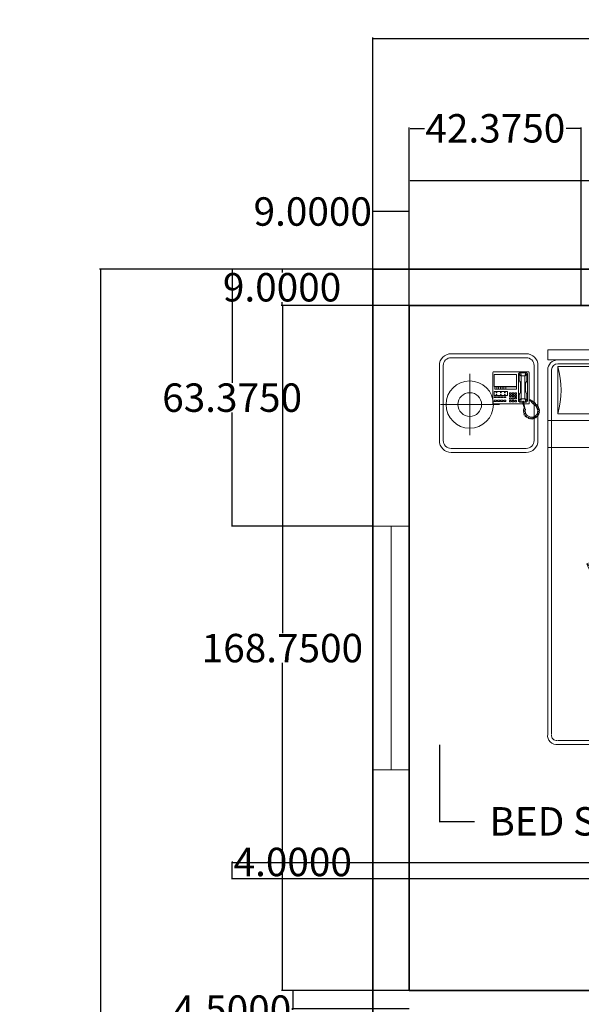
# Model space of a CAD drawing. Units: inches. Extents: x 774 to 2194, y 522 to 1247.
# Tile 4 of 7: x 774 to 912, y 870 to 1112. Entities that reach past the tile are written whole.
import ezdxf

# ---------------------------------------------------------------- set-up
doc = ezdxf.new("R2010")
doc.units = ezdxf.units.IN
for name, color, linetype, lineweight in [('A-ANNO-DIMS', 2, 'Continuous', 13), ('A-FURN', 8, 'Continuous', 18), ('A-GLAZ', 4, 'Continuous', 18), ('A-WALL', 7, 'Continuous', 35)]:
    doc.layers.add(name, color=color, linetype=linetype, lineweight=lineweight)
doc.styles.get("Standard").update_dxf_attribs({"font": 'arial.ttf'})
doc.dimstyles.get("Standard").update_dxf_attribs({"dimtxt": 7, "dimasz": 0.18, "dimexe": 0.18, "dimexo": 0.0625, "dimgap": 0.09, "dimtad": 0, "dimtih": 1, "dimtoh": 1, "dimdec": 4, "dimzin": 0, "dimdsep": 46, "dimtxsty": 'Standard', "dimcen": 0.09, "dimadec": 0, "dimazin": 0, "dimtfac": 1, "dimtdec": 4, "dimtofl": 0, "dimtmove": 0, "dimatfit": 3, "dimfxl": 1, "dimtolj": 1, "dimtzin": 0, "dimarcsym": 0})

# ---------------------------------------------------------------- blocks, each defined once
blk = doc.blocks.new('A$C356F0359')
for p, q in [((0.5489, 2), (2.0492, 2)), ((0.5489, 1.9489), (0.5489, 2)), ((2.0492, 1.9489), (2.0492, 2)), ((0.4398, 1.9801), (0.0598, 1.9801)), ((0.4398, 1.9601), (0.0598, 1.9601)), ((2.0492, 1.9489), (0.5489, 1.9489)), ((2.5283, 1.9801), (2.1483, 1.9801)), ((2.5283, 1.9601), (2.1483, 1.9601)), ((-0.0002, 1.9201), (-0.0002, 1.5401)), ((0.0198, 1.9201), (0.0198, 1.5401)), ((0.4798, 1.5401), (0.4798, 1.9201)), ((0.4998, 1.5401), (0.4998, 1.9201)), ((0.5489, 1.8977), (0.5489, 0.0512)), ((0.5689, 1.8977), (0.5689, 0.0512)), ((1.998, 1.9289), (0.6001, 1.9289)), ((2.0292, 0.0512), (2.0292, 1.8977)), ((2.0492, 0.0512), (2.0492, 1.8977)), ((2.0883, 1.9201), (2.0883, 1.5401)), ((2.1083, 1.9201), (2.1083, 1.5401)), ((2.5683, 1.5401), (2.5683, 1.9201)), ((2.5883, 1.5401), (2.5883, 1.9201)), ((0.1539, 1.5681), (0.1539, 1.8777)), ((0.2725, 1.8879), (0.2702, 1.8856)), ((0.2702, 1.8856), (0.2702, 1.7279)), ((0.2725, 1.8879), (0.4531, 1.8879)), ((0.3913, 1.8753), (0.277, 1.8753)), ((0.277, 1.8753), (0.277, 1.8147)), ((0.3913, 1.8147), (0.3913, 1.8753)), ((0.4016, 1.8787), (0.4062, 1.8845)), ((0.4016, 1.7404), (0.4016, 1.8787)), ((0.4062, 1.881), (0.405, 1.8765)), ((0.405, 1.8765), (0.4153, 1.8662)), ((0.405, 1.8765), (0.405, 1.8456)), ((0.4062, 1.8845), (0.4405, 1.8845)), ((0.4108, 1.8833), (0.4062, 1.881)), ((0.4108, 1.8833), (0.4382, 1.8833)), ((0.4165, 1.8685), (0.4108, 1.8833)), ((0.4153, 1.8662), (0.4165, 1.8685)), ((0.4153, 1.8147), (0.4153, 1.8662)), ((0.4325, 1.8685), (0.4165, 1.8685)), ((0.4325, 1.8685), (0.4382, 1.8833)), ((0.4336, 1.8662), (0.4325, 1.8685)), ((0.4439, 1.8765), (0.4336, 1.8662)), ((0.4336, 1.8147), (0.4336, 1.8662)), ((0.4382, 1.8833), (0.4428, 1.881)), ((0.4405, 1.8845), (0.4462, 1.8787)), ((0.4428, 1.881), (0.4439, 1.8765)), ((0.4439, 1.8765), (0.4439, 1.8456)), ((0.4462, 1.8787), (0.4462, 1.7416)), ((0.4531, 1.8879), (0.4553, 1.8856)), ((0.4553, 1.8856), (0.4553, 1.7279)), ((2.3306, 1.5822), (2.3306, 1.8917)), ((0.277, 1.8147), (0.3913, 1.8147)), ((0.3913, 1.8125), (0.2816, 1.8125)), ((0.2816, 1.8125), (0.2816, 1.801)), ((0.2816, 1.801), (0.3913, 1.801)), ((0.2907, 1.8125), (0.2907, 1.801)), ((0.2999, 1.8125), (0.2999, 1.801)), ((0.309, 1.8125), (0.309, 1.801)), ((0.3182, 1.8125), (0.3182, 1.801)), ((0.3273, 1.8125), (0.3273, 1.801)), ((0.3365, 1.8125), (0.3365, 1.801)), ((0.3913, 1.801), (0.3913, 1.8125)), ((0.405, 1.8456), (0.4073, 1.8399)), ((0.4073, 1.8399), (0.4108, 1.8342)), ((0.4108, 1.8342), (0.4119, 1.8262)), ((0.4119, 1.8262), (0.4119, 1.8147)), ((0.4119, 1.793), (0.4119, 1.8147)), ((0.4153, 1.8147), (0.4153, 1.753)), ((0.4336, 1.8147), (0.4336, 1.753)), ((0.4382, 1.8342), (0.4371, 1.8262)), ((0.4371, 1.8262), (0.4371, 1.8147)), ((0.4371, 1.793), (0.4371, 1.8147)), ((0.4416, 1.8399), (0.4382, 1.8342)), ((0.4439, 1.8456), (0.4416, 1.8399)), ((0.277, 1.7885), (0.277, 1.7679)), ((0.3445, 1.7885), (0.277, 1.7885)), ((0.277, 1.7679), (0.3445, 1.7679)), ((0.2782, 1.7622), (0.2782, 1.7576)), ((0.2896, 1.7622), (0.2782, 1.7622)), ((0.2782, 1.7576), (0.2896, 1.7576)), ((0.2885, 1.7862), (0.2885, 1.7827)), ((0.2919, 1.7862), (0.2885, 1.7862)), ((0.2885, 1.7827), (0.2919, 1.7827)), ((0.2919, 1.7736), (0.2885, 1.7736)), ((0.2885, 1.7736), (0.2885, 1.7702)), ((0.2885, 1.7702), (0.2919, 1.7702)), ((0.2896, 1.7576), (0.2896, 1.7622)), ((0.2919, 1.7827), (0.2919, 1.7862)), ((0.2919, 1.7702), (0.2919, 1.7736)), ((0.2942, 1.7622), (0.2942, 1.7576)), ((0.3056, 1.7622), (0.2942, 1.7622)), ((0.2942, 1.7576), (0.3056, 1.7576)), ((0.3056, 1.7576), (0.3056, 1.7622)), ((0.3125, 1.7862), (0.309, 1.7862)), ((0.309, 1.7862), (0.309, 1.7827)), ((0.309, 1.7827), (0.3125, 1.7827)), ((0.3125, 1.7736), (0.309, 1.7736)), ((0.309, 1.7736), (0.309, 1.7702)), ((0.309, 1.7702), (0.3125, 1.7702)), ((0.3102, 1.7622), (0.3102, 1.7576)), ((0.3216, 1.7622), (0.3102, 1.7622)), ((0.3102, 1.7576), (0.3216, 1.7576)), ((0.3125, 1.7827), (0.3125, 1.7862)), ((0.3125, 1.7702), (0.3125, 1.7736)), ((0.3216, 1.7576), (0.3216, 1.7622)), ((0.3376, 1.7622), (0.3262, 1.7622)), ((0.3262, 1.7622), (0.3262, 1.7576)), ((0.3262, 1.7576), (0.3376, 1.7576)), ((0.333, 1.7862), (0.3296, 1.7862)), ((0.3296, 1.7862), (0.3296, 1.7827)), ((0.3296, 1.7827), (0.333, 1.7827)), ((0.333, 1.7736), (0.3296, 1.7736)), ((0.3296, 1.7736), (0.3296, 1.7702)), ((0.3296, 1.7702), (0.333, 1.7702)), ((0.333, 1.7827), (0.333, 1.7862)), ((0.333, 1.7702), (0.333, 1.7736)), ((0.3376, 1.7576), (0.3376, 1.7622)), ((0.3445, 1.7679), (0.3445, 1.7885)), ((0.3548, 1.7759), (0.3548, 1.7827)), ((0.3548, 1.7827), (0.3639, 1.7827)), ((0.3639, 1.7759), (0.3548, 1.7759)), ((0.3548, 1.7633), (0.3548, 1.7702)), ((0.3548, 1.7702), (0.3639, 1.7702)), ((0.3639, 1.7633), (0.3548, 1.7633)), ((0.3548, 1.7564), (0.3639, 1.7564)), ((0.3548, 1.7496), (0.3548, 1.7564)), ((0.3639, 1.7496), (0.3548, 1.7496)), ((0.3639, 1.7827), (0.3639, 1.7759)), ((0.3639, 1.7702), (0.3639, 1.7633)), ((0.3639, 1.7564), (0.3639, 1.7496)), ((0.3685, 1.7827), (0.3776, 1.7827)), ((0.3685, 1.7759), (0.3685, 1.7827)), ((0.3776, 1.7759), (0.3685, 1.7759)), ((0.3685, 1.7633), (0.3685, 1.7702)), ((0.3685, 1.7702), (0.3776, 1.7702)), ((0.3776, 1.7633), (0.3685, 1.7633)), ((0.3685, 1.7564), (0.3776, 1.7564)), ((0.3685, 1.7496), (0.3685, 1.7564)), ((0.3776, 1.7496), (0.3685, 1.7496)), ((0.3776, 1.7827), (0.3776, 1.7759)), ((0.3776, 1.7702), (0.3776, 1.7633)), ((0.3776, 1.7564), (0.3776, 1.7496)), ((0.3822, 1.7759), (0.3822, 1.7827)), ((0.3822, 1.7827), (0.3913, 1.7827)), ((0.3913, 1.7759), (0.3822, 1.7759)), ((0.3822, 1.7633), (0.3822, 1.7702)), ((0.3822, 1.7702), (0.3913, 1.7702)), ((0.3913, 1.7633), (0.3822, 1.7633)), ((0.3822, 1.7576), (0.3913, 1.7576)), ((0.3822, 1.7507), (0.3822, 1.7576)), ((0.3913, 1.7507), (0.3822, 1.7507)), ((0.3913, 1.7827), (0.3913, 1.7759)), ((0.3913, 1.7702), (0.3913, 1.7633)), ((0.3913, 1.7576), (0.3913, 1.7507)), ((0.405, 1.7736), (0.4073, 1.7793)), ((0.405, 1.7427), (0.405, 1.7736)), ((0.405, 1.7427), (0.4153, 1.753)), ((0.4073, 1.7793), (0.4108, 1.785)), ((0.4108, 1.785), (0.4119, 1.793)), ((0.4165, 1.7507), (0.4108, 1.7359)), ((0.4153, 1.753), (0.4165, 1.7507)), ((0.4325, 1.7507), (0.4165, 1.7507)), ((0.4336, 1.753), (0.4325, 1.7507)), ((0.4325, 1.7507), (0.4382, 1.7359)), ((0.4439, 1.7427), (0.4336, 1.753)), ((0.4382, 1.785), (0.4371, 1.793)), ((0.4416, 1.7793), (0.4382, 1.785)), ((0.4439, 1.7736), (0.4416, 1.7793)), ((0.4439, 1.7427), (0.4439, 1.7736)), ((0.4622, 1.7459), (0.4553, 1.7484)), ((0.3052, 1.7226), (0.0051, 1.7226)), ((0.2702, 1.7279), (0.2725, 1.7256)), ((0.4244, 1.7256), (0.2725, 1.7256)), ((0.2782, 1.745), (0.2896, 1.745)), ((0.2782, 1.7382), (0.2782, 1.745)), ((0.2896, 1.7382), (0.2782, 1.7382)), ((0.2896, 1.745), (0.2896, 1.7382)), ((0.2942, 1.745), (0.3056, 1.745)), ((0.2942, 1.7382), (0.2942, 1.745)), ((0.3056, 1.7382), (0.2942, 1.7382)), ((0.3056, 1.745), (0.3056, 1.7382)), ((0.3102, 1.745), (0.3216, 1.745)), ((0.3102, 1.7382), (0.3102, 1.745)), ((0.3216, 1.7382), (0.3102, 1.7382)), ((0.3216, 1.745), (0.3216, 1.7382)), ((0.3262, 1.7382), (0.3262, 1.745)), ((0.3262, 1.745), (0.3376, 1.745)), ((0.3376, 1.7382), (0.3262, 1.7382)), ((0.3376, 1.745), (0.3376, 1.7382)), ((0.3548, 1.737), (0.3548, 1.7439)), ((0.3548, 1.7439), (0.3639, 1.7439)), ((0.3639, 1.737), (0.3548, 1.737)), ((0.3639, 1.7439), (0.3639, 1.737)), ((0.3685, 1.737), (0.3685, 1.7439)), ((0.3685, 1.7439), (0.3776, 1.7439)), ((0.3776, 1.737), (0.3685, 1.737)), ((0.3776, 1.7439), (0.3776, 1.737)), ((0.3822, 1.7439), (0.3913, 1.7439)), ((0.3822, 1.737), (0.3822, 1.7439)), ((0.3913, 1.737), (0.3822, 1.737)), ((0.3913, 1.7439), (0.3913, 1.737)), ((0.4073, 1.7347), (0.4016, 1.7404)), ((0.4062, 1.7382), (0.405, 1.7427)), ((0.4108, 1.7359), (0.4062, 1.7382)), ((0.4234, 1.7347), (0.4073, 1.7347)), ((0.4108, 1.7359), (0.4234, 1.7359)), ((0.4233, 1.7393), (0.4235, 1.7294)), ((0.4268, 1.7393), (0.4233, 1.7393)), ((0.4235, 1.7294), (0.4263, 1.7179)), ((0.4263, 1.7179), (0.429, 1.707)), ((0.427, 1.697), (0.4265, 1.6915)), ((0.4274, 1.7301), (0.4268, 1.7393)), ((0.427, 1.7359), (0.4382, 1.7359)), ((0.4295, 1.6996), (0.427, 1.697)), ((0.4405, 1.7347), (0.4271, 1.7347)), ((0.429, 1.7227), (0.4274, 1.7301)), ((0.4531, 1.7256), (0.4284, 1.7256)), ((0.429, 1.707), (0.4288, 1.701)), ((0.4288, 1.701), (0.4295, 1.6996)), ((0.4318, 1.7119), (0.429, 1.7227)), ((0.4325, 1.7063), (0.4318, 1.7119)), ((0.4323, 1.7003), (0.4325, 1.7063)), ((0.4364, 1.6973), (0.4323, 1.7003)), ((0.4355, 1.6919), (0.4364, 1.6973)), ((0.4382, 1.7359), (0.4428, 1.7382)), ((0.4462, 1.7416), (0.4405, 1.7347)), ((0.4428, 1.7382), (0.4439, 1.7427)), ((0.4553, 1.7279), (0.4531, 1.7256)), ((0.4553, 1.7439), (0.4604, 1.7425)), ((0.4604, 1.7425), (0.465, 1.7388)), ((0.4654, 1.7427), (0.4622, 1.7459)), ((0.465, 1.7388), (0.4662, 1.7372)), ((0.4678, 1.7405), (0.4654, 1.7427)), ((0.4662, 1.7372), (0.4686, 1.7374)), ((0.4686, 1.7374), (0.4662, 1.735)), ((0.4662, 1.735), (0.4755, 1.7268)), ((0.4721, 1.7421), (0.4678, 1.7405)), ((0.4741, 1.7401), (0.4721, 1.7421)), ((0.4725, 1.7366), (0.4741, 1.7401)), ((0.4753, 1.7388), (0.4725, 1.7366)), ((0.4783, 1.7356), (0.4753, 1.7388)), ((0.4755, 1.7268), (0.4906, 1.7139)), ((0.4759, 1.729), (0.4783, 1.7356)), ((0.4821, 1.7322), (0.4759, 1.729)), ((0.4874, 1.7272), (0.4821, 1.7322)), ((0.4862, 1.7199), (0.4874, 1.7272)), ((0.4914, 1.7231), (0.4862, 1.7199)), ((0.4908, 1.7135), (0.4984, 1.6917)), ((0.4958, 1.7185), (0.4914, 1.7231)), ((0.494, 1.7135), (0.4958, 1.7185)), ((0.501, 1.7142), (0.494, 1.7135)), ((0.4964, 1.7047), (0.5031, 1.7072)), ((0.5038, 1.7049), (0.4964, 1.7047)), ((0.5005, 1.695), (0.5054, 1.6996)), ((0.5031, 1.7072), (0.501, 1.7142)), ((0.5054, 1.6996), (0.5038, 1.7049)), ((2.4819, 1.7366), (2.1818, 1.7366)), ((0.4265, 1.6915), (0.4332, 1.6903)), ((0.4332, 1.6903), (0.4267, 1.6864)), ((0.4267, 1.6864), (0.4272, 1.6801)), ((0.4272, 1.6801), (0.4346, 1.6794)), ((0.4346, 1.6794), (0.4281, 1.6744)), ((0.4281, 1.6744), (0.4311, 1.669)), ((0.4311, 1.669), (0.4381, 1.6704)), ((0.4381, 1.6704), (0.4348, 1.6639)), ((0.4348, 1.6639), (0.4383, 1.6598)), ((0.4367, 1.6774), (0.4355, 1.6919)), ((0.4455, 1.6663), (0.4367, 1.6774)), ((0.4383, 1.6598), (0.4436, 1.6637)), ((0.4436, 1.6637), (0.4427, 1.6575)), ((0.4427, 1.6575), (0.4471, 1.6547)), ((0.4577, 1.6598), (0.4455, 1.6663)), ((0.4471, 1.6547), (0.4526, 1.6593)), ((0.4526, 1.6593), (0.4519, 1.6517)), ((0.4519, 1.6517), (0.4568, 1.6503)), ((0.4568, 1.6503), (0.4598, 1.6565)), ((0.4716, 1.6586), (0.4577, 1.6598)), ((0.4598, 1.6565), (0.4626, 1.6503)), ((0.4626, 1.6503), (0.4665, 1.6498)), ((0.4665, 1.6498), (0.4681, 1.6565)), ((0.4681, 1.6565), (0.4707, 1.6491)), ((0.4707, 1.6491), (0.4751, 1.6503)), ((0.485, 1.6644), (0.4716, 1.6586)), ((0.4751, 1.6503), (0.4753, 1.6565)), ((0.4753, 1.6565), (0.4806, 1.6519)), ((0.4806, 1.6519), (0.4843, 1.6538)), ((0.4843, 1.6538), (0.4836, 1.6607)), ((0.4836, 1.6607), (0.4885, 1.6547)), ((0.4952, 1.6744), (0.485, 1.6644)), ((0.4885, 1.6547), (0.4922, 1.6579)), ((0.4922, 1.6579), (0.4894, 1.6642)), ((0.4894, 1.6642), (0.4959, 1.6614)), ((0.4984, 1.6917), (0.4952, 1.6744)), ((0.4957, 1.6704), (0.5024, 1.6683)), ((0.4989, 1.6642), (0.4957, 1.6704)), ((0.4959, 1.6614), (0.4989, 1.6642)), ((0.5042, 1.673), (0.4987, 1.6792)), ((0.4987, 1.6792), (0.5058, 1.679)), ((0.5068, 1.695), (0.5005, 1.695)), ((0.5008, 1.6871), (0.5079, 1.6892)), ((0.5068, 1.6836), (0.5008, 1.6871)), ((0.5024, 1.6683), (0.5042, 1.673)), ((0.5058, 1.679), (0.5068, 1.6836)), ((0.5079, 1.6892), (0.5068, 1.695)), ((0.0598, 1.5001), (0.4398, 1.5001)), ((2.1483, 1.5001), (2.5283, 1.5001)), ((0.0598, 1.4801), (0.4398, 1.4801)), ((2.1483, 1.4801), (2.5283, 1.4801)), ((0.6001, 0.02), (1.998, 0.02)), ((0.6001, 0), (1.998, 0))]:
    blk.add_line(p, q)
at = {"linetype": 'ByBlock'}
for p, q in [((0.6001, 1.9147), (1.282, 1.9147)), ((0.6001, 1.6759), (0.6001, 1.9147)), ((1.282, 1.9147), (1.282, 1.6759)), ((1.3161, 1.9147), (1.998, 1.9147)), ((1.3161, 1.6759), (1.3161, 1.9147)), ((1.998, 1.9147), (1.998, 1.6759)), ((1.282, 1.6759), (0.6001, 1.6759)), ((1.998, 1.6759), (1.3161, 1.6759)), ((1.0687, 1.6418), (0.5489, 1.6418)), ((1.4185, 1.5053), (0.5489, 1.5053))]:
    blk.add_line(p, q, dxfattribs=at)
for centre in [(2.3306, 1.7366), (0.1539, 1.7226)]:
    blk.add_circle(centre, 0.12, dxfattribs=at)
for centre in [(2.3306, 1.7366), (0.1539, 1.7226)]:
    blk.add_circle(centre, 0.06)
for centre, radius, start, end in [((0.0598, 1.9201), 0.06, 90, 180), ((0.0598, 1.9201), 0.04, 90, 180), ((0.4398, 1.9201), 0.06, 0, 90), ((0.4398, 1.9201), 0.04, 0, 90), ((0.6001, 1.8977), 0.0512, 90, 180), ((1.998, 1.8977), 0.0512, 0, 90), ((2.1483, 1.9201), 0.06, 90, 180), ((2.1483, 1.9201), 0.04, 90, 180), ((2.5283, 1.9201), 0.06, 0, 90), ((2.5283, 1.9201), 0.04, 0, 90), ((0.6001, 1.8977), 0.0312, 90, 180), ((1.998, 1.8977), 0.0312, 0, 90), ((0.0598, 1.5401), 0.06, 180, 270), ((0.0598, 1.5401), 0.04, 180, 270), ((0.4398, 1.5401), 0.04, 270, 0), ((0.4398, 1.5401), 0.06, 270, 0), ((2.1483, 1.5401), 0.06, 180, 270), ((2.1483, 1.5401), 0.04, 180, 270), ((2.5283, 1.5401), 0.06, 270, 0), ((2.5283, 1.5401), 0.04, 270, 0), ((1.1471, 0.7332), 0.3575, 102.4782, 140.4625), ((1.9086, 1.3124), 0.8697, 195.336, 226.4193), ((0.3249, 0.4335), 0.9879, 28.4971, 41.0566), ((0.9965, 0.4273), 0.548, 103.2034, 117.0362), ((1.6529, 1.7059), 1.0798, 223.6306, 251.4288), ((0.4451, 0.4375), 0.5655, 5.3391, 57.6895), ((0.4517, 0.5274), 0.4879, 10.6986, 52.6864), ((1.8195, 1.3719), 1.1652, 203.0642, 220.3209), ((0.5617, 0.4344), 0.7874, 18.3527, 36.6851), ((-0.021, 2.4319), 2.1977, 305.2966, 307.2418), ((1.5949, 0.9312), 0.734, 205.259, 216.9351), ((1.4135, 0.487), 0.3575, 154.0418, 192.0262), ((1.3641, 0.0041), 0.6085, 71.81, 120.1351), ((1.1372, -0.3434), 0.9879, 80.0607, 92.6202), ((1.2836, -0.1573), 0.7874, 69.9163, 88.2487), ((1.44, 0.1186), 0.4774, 76.1849, 142.0017), ((-0.6432, 0.628), 2.1977, 349.4884, 358.8054), ((-0.021, 2.4319), 2.1977, 297.9248, 299.3793), ((1.5595, 0.1789), 0.548, 154.767, 168.5998), ((1.2647, 0.9578), 0.6885, 250.2936, 293.6414), ((1.3312, 1.4107), 1.1652, 254.6278, 271.8845), ((1.5368, 0.9609), 0.734, 256.8226, 268.4988), ((0.5943, 0.0454), 0.0458, 172.7599, 277.2401), ((2.0038, 0.0454), 0.0458, 262.7599, 7.2401), ((0.5943, 0.0454), 0.0258, 172.7599, 277.2401), ((2.0038, 0.0454), 0.0258, 262.7599, 7.2401)]:
    blk.add_arc(centre, radius, start, end)
for centre, radius, start, end in [((0.1906, 1.7953), 0.4265, 343.7398, 16.2602), ((1.6914, 1.7953), 0.4265, 163.7398, 196.2602), ((0.9067, 1.7953), 0.4265, 343.7398, 16.2602), ((2.4075, 1.7953), 0.4265, 163.7398, 196.2602), ((0.9303, 0.657), 0.9853, 61.4328, 88.1261), ((1.0826, 0.5712), 1.0706, 72.1966, 90.7418), ((2.1368, 4.5996), 3.0955, 256.4201, 268.3789), ((2.0056, 2.7745), 1.3903, 244.2427, 271.7984)]:
    blk.add_arc(centre, radius, start, end, dxfattribs=at)
blk = doc.blocks.new('*D9')
at = {"layer": 'A-ANNO-DIMS', "color": 0, "lineweight": -2, "transparency": 16777216}
for p, q in [((860.78, 1064.85), (860.6, 1064.85)), ((860.78, 1041.75), (860.78, 1065.03)), ((869.6, 1064.85), (860.96, 1064.85)), ((869.78, 1041.75), (869.78, 1065.03))]:
    blk.add_line(p, q, dxfattribs=at)
at = {"layer": 'A-ANNO-DIMS', "color": 0, "transparency": 16777216}
for points in [[(860.96, 1064.88), (860.96, 1064.82), (860.78, 1064.85)], [(869.6, 1064.88), (869.6, 1064.82), (869.78, 1064.85)]]:
    blk.add_solid(points, dxfattribs=at)
at = {"layer": 'Defpoints', "color": 0, "transparency": 16777216}
for p in [(860.78, 1064.85), (860.78, 1041.69), (869.78, 1041.69)]:
    blk.add_point(p, dxfattribs=at)
at = {"layer": 'A-ANNO-DIMS', "color": 0, "transparency": 16777216, "insert": (845.99, 1064.85), "char_height": 7, "attachment_point": 5}
blk.add_mtext('\\A1;9.0000', dxfattribs=at)
blk = doc.blocks.new('*D10')
at = {"layer": 'A-ANNO-DIMS', "color": 0, "lineweight": -2, "transparency": 16777216}
for p, q in [((869.78, 1041.75), (869.78, 1072.68)), ((869.96, 1072.5), (922.44, 1072.5)), ((1014.35, 1072.5), (961.87, 1072.5)), ((1014.53, 1041.75), (1014.53, 1072.68))]:
    blk.add_line(p, q, dxfattribs=at)
at = {"layer": 'A-ANNO-DIMS', "color": 0, "transparency": 16777216}
for points in [[(869.96, 1072.53), (869.96, 1072.47), (869.78, 1072.5)], [(1014.35, 1072.53), (1014.35, 1072.47), (1014.53, 1072.5)]]:
    blk.add_solid(points, dxfattribs=at)
at = {"layer": 'Defpoints', "color": 0, "transparency": 16777216}
for p in [(1014.53, 1072.5), (869.78, 1041.69), (1014.53, 1041.69)]:
    blk.add_point(p, dxfattribs=at)
at = {"layer": 'A-ANNO-DIMS', "color": 0, "transparency": 16777216, "insert": (942.16, 1072.5), "char_height": 7, "attachment_point": 5}
blk.add_mtext('\\A1;144.7500', dxfattribs=at)
blk = doc.blocks.new('*D15')
at = {"layer": 'A-ANNO-DIMS', "color": 0, "lineweight": -2, "transparency": 16777216}
for p, q in [((860.78, 1053.45), (860.78, 1107.69)), ((860.96, 1107.51), (1020.74, 1107.51)), ((1220.6, 1107.51), (1060.83, 1107.51)), ((1220.78, 1050.75), (1220.78, 1107.69))]:
    blk.add_line(p, q, dxfattribs=at)
at = {"layer": 'A-ANNO-DIMS', "color": 0, "transparency": 16777216}
for points in [[(860.96, 1107.54), (860.96, 1107.48), (860.78, 1107.51)], [(1220.6, 1107.54), (1220.6, 1107.48), (1220.78, 1107.51)]]:
    blk.add_solid(points, dxfattribs=at)
at = {"layer": 'Defpoints', "color": 0, "transparency": 16777216}
for p in [(1220.78, 1107.51), (860.78, 1053.39), (1220.78, 1050.69)]:
    blk.add_point(p, dxfattribs=at)
at = {"layer": 'A-ANNO-DIMS', "color": 0, "transparency": 16777216, "insert": (1040.78, 1107.51), "char_height": 7, "attachment_point": 5}
blk.add_mtext('\\A1;360.0000', dxfattribs=at)
blk = doc.blocks.new('*D16')
at = {"layer": 'A-ANNO-DIMS', "color": 0, "lineweight": -2, "transparency": 16777216}
for p, q in [((869.72, 1050.69), (838.25, 1050.69)), ((838.43, 1050.51), (838.43, 1049.85)), ((869.72, 1041.69), (838.25, 1041.69)), ((838.43, 1041.87), (838.43, 1042.52))]:
    blk.add_line(p, q, dxfattribs=at)
at = {"layer": 'A-ANNO-DIMS', "color": 0, "transparency": 16777216}
for points in [[(838.4, 1050.51), (838.46, 1050.51), (838.43, 1050.69)], [(838.4, 1041.87), (838.46, 1041.87), (838.43, 1041.69)]]:
    blk.add_solid(points, dxfattribs=at)
at = {"layer": 'Defpoints', "color": 0, "transparency": 16777216}
for p in [(869.78, 1050.69), (838.43, 1041.69), (869.78, 1041.69)]:
    blk.add_point(p, dxfattribs=at)
at = {"layer": 'A-ANNO-DIMS', "color": 0, "transparency": 16777216, "insert": (838.43, 1046.19), "char_height": 7, "attachment_point": 5}
blk.add_mtext('\\A1;9.0000', dxfattribs=at)
blk = doc.blocks.new('*D17')
at = {"layer": 'A-ANNO-DIMS', "color": 0, "lineweight": -2, "transparency": 16777216}
for p, q in [((869.72, 1041.69), (838.33, 1041.69)), ((838.51, 1041.51), (838.51, 960.98)), ((838.51, 873.12), (838.51, 953.65)), ((869.72, 872.94), (838.33, 872.94))]:
    blk.add_line(p, q, dxfattribs=at)
at = {"layer": 'A-ANNO-DIMS', "color": 0, "transparency": 16777216}
for points in [[(838.48, 1041.51), (838.54, 1041.51), (838.51, 1041.69)], [(838.48, 873.12), (838.54, 873.12), (838.51, 872.94)]]:
    blk.add_solid(points, dxfattribs=at)
at = {"layer": 'Defpoints', "color": 0, "transparency": 16777216}
for p in [(869.78, 1041.69), (838.51, 872.94), (869.78, 872.94)]:
    blk.add_point(p, dxfattribs=at)
at = {"layer": 'A-ANNO-DIMS', "color": 0, "transparency": 16777216, "insert": (838.51, 957.31), "char_height": 7, "attachment_point": 5}
blk.add_mtext('\\A1;168.7500', dxfattribs=at)
blk = doc.blocks.new('*D18')
at = {"layer": 'A-ANNO-DIMS', "color": 0, "lineweight": -2, "transparency": 16777216}
for p, q in [((869.72, 872.94), (840.87, 872.94)), ((841.05, 872.76), (841.05, 868.62)), ((869.72, 868.44), (840.87, 868.44)), ((841.05, 868.44), (841.05, 868.26)), ((841.05, 868.26), (840.87, 868.26))]:
    blk.add_line(p, q, dxfattribs=at)
at = {"layer": 'A-ANNO-DIMS', "color": 0, "transparency": 16777216}
for points in [[(841.02, 872.76), (841.08, 872.76), (841.05, 872.94)], [(841.02, 868.62), (841.08, 868.62), (841.05, 868.44)]]:
    blk.add_solid(points, dxfattribs=at)
at = {"layer": 'Defpoints', "color": 0, "transparency": 16777216}
for p in [(869.78, 872.94), (841.05, 868.44), (869.78, 868.44)]:
    blk.add_point(p, dxfattribs=at)
at = {"layer": 'A-ANNO-DIMS', "color": 0, "transparency": 16777216, "insert": (826.12, 868.26), "char_height": 7, "attachment_point": 5}
blk.add_mtext('\\A1;4.5000', dxfattribs=at)
blk = doc.blocks.new('*D22')
at = {"layer": 'A-ANNO-DIMS', "color": 0, "lineweight": -2, "transparency": 16777216}
for p, q in [((869.72, 1050.69), (793.49, 1050.69)), ((793.67, 1050.51), (793.67, 809.85)), ((793.67, 561.87), (793.67, 802.52)), ((869.72, 561.69), (793.49, 561.69))]:
    blk.add_line(p, q, dxfattribs=at)
at = {"layer": 'A-ANNO-DIMS', "color": 0, "transparency": 16777216}
for points in [[(793.64, 1050.51), (793.7, 1050.51), (793.67, 1050.69)], [(793.64, 561.87), (793.7, 561.87), (793.67, 561.69)]]:
    blk.add_solid(points, dxfattribs=at)
at = {"layer": 'Defpoints', "color": 0, "transparency": 16777216}
for p in [(869.78, 1050.69), (793.67, 561.69), (869.78, 561.69)]:
    blk.add_point(p, dxfattribs=at)
at = {"layer": 'A-ANNO-DIMS', "color": 0, "transparency": 16777216, "insert": (793.67, 806.19), "char_height": 7, "attachment_point": 5}
blk.add_mtext('\\A1;489.0000', dxfattribs=at)
blk = doc.blocks.new('WIN-60IN-EXT')
for p, q in [((0, 0), (0, 9)), ((60, 0), (60, 9)), ((0, 4.5), (60, 4.5))]:
    blk.add_line(p, q)
blk = doc.blocks.new('*D42')
at = {"layer": 'A-ANNO-DIMS', "color": 0, "lineweight": -2, "transparency": 16777216}
for p, q in [((877.18, 933.44), (877.18, 914.45)), ((1002.99, 933.44), (1002.99, 914.45)), ((877.36, 914.63), (885.88, 914.63)), ((1002.81, 914.63), (994.29, 914.63))]:
    blk.add_line(p, q, dxfattribs=at)
at = {"layer": 'A-ANNO-DIMS', "color": 0, "transparency": 16777216}
for points in [[(877.36, 914.66), (877.36, 914.6), (877.18, 914.63)], [(1002.81, 914.66), (1002.81, 914.6), (1002.99, 914.63)]]:
    blk.add_solid(points, dxfattribs=at)
at = {"layer": 'Defpoints', "color": 0, "transparency": 16777216}
for p in [(877.18, 933.5), (1002.99, 933.5), (1002.99, 914.63)]:
    blk.add_point(p, dxfattribs=at)
at = {"layer": 'A-ANNO-DIMS', "color": 0, "transparency": 16777216, "insert": (940.09, 914.63), "char_height": 7, "attachment_point": 5}
blk.add_mtext('\\A1;BED SET 125.8041 TYP.', dxfattribs=at)
blk = doc.blocks.new('*D58')
at = {"layer": 'A-ANNO-DIMS', "color": 0, "lineweight": -2, "transparency": 16777216}
for p, q in [((869.78, 1041.75), (869.78, 1085.52)), ((869.96, 1085.34), (873.5, 1085.34)), ((911.98, 1085.34), (908.44, 1085.34)), ((912.16, 1041.75), (912.16, 1085.52))]:
    blk.add_line(p, q, dxfattribs=at)
at = {"layer": 'A-ANNO-DIMS', "color": 0, "transparency": 16777216}
for points in [[(869.96, 1085.37), (869.96, 1085.31), (869.78, 1085.34)], [(911.98, 1085.37), (911.98, 1085.31), (912.16, 1085.34)]]:
    blk.add_solid(points, dxfattribs=at)
at = {"layer": 'Defpoints', "color": 0, "transparency": 16777216}
for p in [(912.16, 1085.34), (869.78, 1041.69), (912.16, 1041.69)]:
    blk.add_point(p, dxfattribs=at)
at = {"layer": 'A-ANNO-DIMS', "color": 0, "transparency": 16777216, "insert": (890.97, 1085.34), "char_height": 7, "attachment_point": 5}
blk.add_mtext('\\A1;42.3750', dxfattribs=at)
blk = doc.blocks.new('*D61')
at = {"layer": 'A-ANNO-DIMS', "color": 0, "lineweight": -2, "transparency": 16777216}
for p, q in [((860.72, 1050.69), (825.95, 1050.69)), ((826.13, 1050.51), (826.13, 1022.67)), ((826.13, 987.49), (826.13, 1015.33)), ((860.72, 987.31), (825.95, 987.31))]:
    blk.add_line(p, q, dxfattribs=at)
at = {"layer": 'A-ANNO-DIMS', "color": 0, "transparency": 16777216}
for points in [[(826.1, 1050.51), (826.16, 1050.51), (826.13, 1050.69)], [(826.1, 987.49), (826.16, 987.49), (826.13, 987.31)]]:
    blk.add_solid(points, dxfattribs=at)
at = {"layer": 'Defpoints', "color": 0, "transparency": 16777216}
for p in [(826.13, 1050.69), (860.78, 1050.69), (860.78, 987.31)]:
    blk.add_point(p, dxfattribs=at)
at = {"layer": 'A-ANNO-DIMS', "color": 0, "transparency": 16777216, "insert": (826.13, 1019), "char_height": 7, "attachment_point": 5}
blk.add_mtext('\\A1;63.3750', dxfattribs=at)
blk = doc.blocks.new('*D72')
at = {"layer": 'A-ANNO-DIMS', "color": 0, "lineweight": -2, "transparency": 16777216}
for p, q in [((1138.97, 904.44), (825.95, 904.44)), ((826.13, 904.44), (826.13, 904.62)), ((826.13, 904.62), (826.31, 904.62)), ((826.13, 900.62), (826.13, 904.26)), ((1138.97, 900.44), (825.95, 900.44))]:
    blk.add_line(p, q, dxfattribs=at)
at = {"layer": 'A-ANNO-DIMS', "color": 0, "transparency": 16777216}
for points in [[(826.1, 904.26), (826.16, 904.26), (826.13, 904.44)], [(826.1, 900.62), (826.16, 900.62), (826.13, 900.44)]]:
    blk.add_solid(points, dxfattribs=at)
at = {"layer": 'Defpoints', "color": 0, "transparency": 16777216}
for p in [(826.13, 904.44), (1139.03, 904.44), (1139.03, 900.44)]:
    blk.add_point(p, dxfattribs=at)
at = {"layer": 'A-ANNO-DIMS', "color": 0, "transparency": 16777216, "insert": (841.06, 904.62), "char_height": 7, "attachment_point": 5}
blk.add_mtext('\\A1;4.0000', dxfattribs=at)

msp = doc.modelspace()

# ---------------------------------------------------------------- linework, layer by layer
at = {"layer": 'A-WALL'}
for p, q in [((1220.78103, 1050.6875), (860.78103, 1050.6875)), ((860.78103, 1050.6875), (860.78103, 561.6875)), ((860.78103, 1050.6875), (1220.78103, 1050.6875)), ((869.78103, 1041.6875), (1014.53103, 1041.6875)), ((869.78103, 1041.6875), (869.78103, 872.9375)), ((869.78103, 1041.6875), (1014.53103, 1041.6875)), ((869.78103, 872.9375), (869.78103, 1041.6875)), ((1014.53103, 1041.6875), (869.78103, 1041.6875)), ((869.78103, 872.9375), (1014.53103, 872.9375))]:
    msp.add_line(p, q, dxfattribs=at)

# ---------------------------------------------------------------- block references
at = {"layer": 'A-FURN', "xscale": 48.60038017161549, "yscale": 48.60038017161549, "zscale": 48.60038017161549}
msp.add_blockref('A$C356F0359', (877.19418, 933.58323), dxfattribs=at)
at = {"layer": 'A-GLAZ', "rotation": 89.9999999999996}
msp.add_blockref('WIN-60IN-EXT', (869.78053, 927.31248), dxfattribs=at)

# ---------------------------------------------------------------- dimensions: what is measured, and where the dimension line sits
at = {"layer": 'A-ANNO-DIMS'}
for base, p1, p2, override, picture, middle in [((1220.78103, 1107.50884), (860.78103, 1053.38824), (1220.78103, 1050.6875), {"dimclrd": 0, "dimclre": 0, "dimclrt": 0}, '*D15', (1040.78103, 1107.50884)), ((912.15603, 1085.3375), (869.78103, 1041.6875), (912.15603, 1041.6875), {"dimdec": 4, "dimlfac": 1, "dimrnd": 0, "dimzin": 0, "dimdsep": 46, "dimlunit": 2}, '*D58', (890.96853, 1085.3375)), ((1014.53103, 1072.49891), (869.78103, 1041.6875), (1014.53103, 1041.6875), {"dimclrd": 0, "dimclre": 0, "dimclrt": 0}, '*D10', (942.15603, 1072.49891)), ((860.78103, 1064.84648), (869.78103, 1041.6875), (860.78103, 1041.6875), {"dimclrd": 0, "dimclre": 0, "dimclrt": 0}, '*D9', (845.99295, 1064.84648))]:
    dim = msp.add_linear_dim(base=base, p1=p1, p2=p2, dimstyle='Standard', override=override, dxfattribs=at)
    dim.commit()
    dim.dimension.update_dxf_attribs({"geometry": picture, "text_midpoint": middle})
for base, p1, p2, override, picture, middle in [((793.67062, 561.6875), (869.78103, 1050.6875), (869.78103, 561.6875), {"dimclrd": 0, "dimclre": 0, "dimclrt": 0}, '*D22', (793.67062, 806.1875)), ((826.13103, 1050.6875), (860.78103, 987.3125), (860.78103, 1050.6875), {"dimdec": 4, "dimlfac": 1, "dimrnd": 0, "dimzin": 0, "dimdsep": 46, "dimlunit": 2}, '*D61', (826.13103, 1019)), ((838.42629, 1041.6875), (869.78103, 1050.6875), (869.78103, 1041.6875), {"dimclrd": 0, "dimclre": 0, "dimclrt": 0}, '*D16', (838.42629, 1046.1875)), ((838.50889, 872.9375), (869.78103, 1041.6875), (869.78103, 872.9375), {"dimclrd": 0, "dimclre": 0, "dimclrt": 0}, '*D17', (838.50889, 957.3125)), ((826.13103, 904.4375), (1139.03103, 900.4375), (1139.03103, 904.4375), {"dimdec": 4, "dimlfac": 1, "dimrnd": 0, "dimzin": 0, "dimdsep": 46, "dimlunit": 2}, '*D72', (841.05996, 904.6175)), ((841.05064, 868.4375), (869.78103, 872.9375), (869.78103, 868.4375), {"dimclrd": 0, "dimclre": 0, "dimclrt": 0}, '*D18', (826.1217, 868.2575))]:
    dim = msp.add_linear_dim(base=base, p1=p1, p2=p2, angle=90, dimstyle='Standard', override=override, dxfattribs=at)
    dim.commit()
    dim.dimension.update_dxf_attribs({"geometry": picture, "text_midpoint": middle})
dim = msp.add_linear_dim(base=(1002.98727, 914.62773), p1=(877.18318, 933.49835), p2=(1002.98727, 933.49835), text='BED SET <> TYP.', dimstyle='Standard', override={"dimdec": 4, "dimlfac": 1, "dimrnd": 0, "dimzin": 0, "dimdsep": 46, "dimlunit": 2}, dxfattribs=at)
dim.commit()
dim.dimension.update_dxf_attribs({"geometry": '*D42', "text_midpoint": (940.08523, 914.62773)})

doc.saveas('drawing.dxf')
